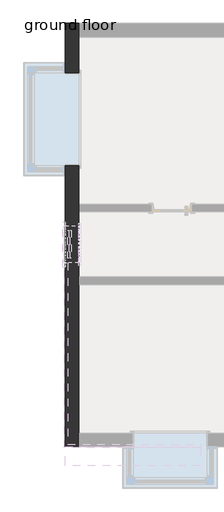
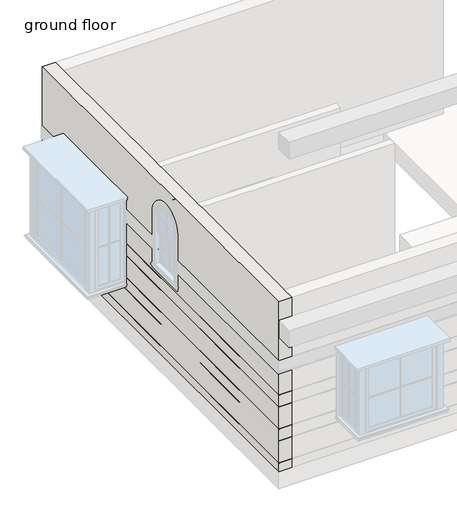
# One storey, part 2 of 5: 1 wall.
"""IFC4 building model written with IfcOpenShell, lengths in millimetres."""

from ifc_helpers import new_model, si_unit, frame, origin, place, context, project, spatial, polyline, circle_curve, ellipse_curve, element, save
from ifc_brep_helpers import plane_surface, cylinder_surface, revolved_surface, advanced_brep

model = new_model("IFC4")

# Units and contexts
model_context = context("Model", 3, world=origin())
ifc_project = project(units=[si_unit("LENGTHUNIT", "METRE", prefix="MILLI")], contexts=[model_context])

# Site, building, storey
site = spatial("IfcSite", under=ifc_project)
building = spatial("IfcBuilding", under=site)
storey = spatial("IfcBuildingStorey", under=building, Name="ground floor", Elevation=304.8)

# Wall
placement = place(None, origin())
element("IfcWall", 1, ObjectType="OUTER WALL 9\"", at=placement, inside=storey, context=model_context, shape_type="AdvancedBrep", body=[
    advanced_brep(
    [(-13179.0672301, -305.6302427, 304.8), (-13179.0672301, -7265.2302427, 304.8), (-13179.0672301, -7265.2302427, 455.95311), (-13179.0672301, -305.6302427, 455.95311), (-13179.0672301, -7265.2302427, 3352.8), (-13179.0672301, -305.6302427, 3352.8), (-13179.0672301, -305.6302427, 2298.7), (-13179.0672301, -1118.4302427, 2298.7), (-13179.0672301, -1118.4302427, 2489.2), (-13179.0672301, -2642.4302427, 2489.2), (-13179.0672301, -2642.4302427, 2298.7), (-13179.0672301, -3633.0302427, 2298.7), (-13179.0672301, -3633.0302427, 2743.2), (-13179.0672301, -4242.6302427, 2743.2), (-13179.0672301, -4242.6302427, 2298.7), (-13179.0672301, -7265.2302427, 2298.7), (-13179.0672301, -2642.4302427, 914.4), (-13179.0672301, -1118.4302427, 914.4), (-13179.0672301, -1118.4302427, 1065.55311), (-13179.0672301, -305.6302427, 1065.55311), (-13179.0672301, -305.6302427, 864.84689), (-13179.0672301, -1118.4302427, 864.84689), (-13179.0672301, -1118.4302427, 850.9), (-13179.0672301, -305.6302427, 850.9), (-13179.0672301, -305.6302427, 469.9), (-13179.0672301, -7265.2302427, 469.9), (-13179.0672301, -7265.2302427, 850.9), (-13179.0672301, -2642.4302427, 850.9), (-13179.0672301, -2642.4302427, 864.84689), (-13179.0672301, -7265.2302427, 864.84689), (-13179.0672301, -7265.2302427, 1065.55311), (-13179.0672301, -2642.4302427, 1065.55311), (-13179.0672301, -4242.6302427, 1828.8), (-13179.0672301, -3633.0302427, 1828.8), (-13179.0672301, -3633.0302427, 2070.1), (-13179.0672301, -2642.4302427, 2070.1), (-13179.0672301, -2642.4302427, 1689.1), (-13179.0672301, -7265.2302427, 1689.1), (-13179.0672301, -7265.2302427, 2070.1), (-13179.0672301, -4242.6302427, 2070.1), (-13179.0672301, -305.6302427, 2284.75311), (-13179.0672301, -305.6302427, 2084.04689), (-13179.0672301, -1118.4302427, 2084.04689), (-13179.0672301, -1118.4302427, 2284.75311), (-13179.0672301, -2642.4302427, 2284.75311), (-13179.0672301, -2642.4302427, 2084.04689), (-13179.0672301, -3633.0302427, 2084.04689), (-13179.0672301, -3633.0302427, 2284.75311), (-13179.0672301, -4242.6302427, 2284.75311), (-13179.0672301, -4242.6302427, 2084.04689), (-13179.0672301, -7265.2302427, 2084.04689), (-13179.0672301, -7265.2302427, 2284.75311), (-13179.0672301, -1118.4302427, 2070.1), (-13179.0672301, -305.6302427, 2070.1), (-13179.0672301, -305.6302427, 1689.1), (-13179.0672301, -1118.4302427, 1689.1), (-13179.0672301, -2642.4302427, 1675.15311), (-13179.0672301, -2642.4302427, 1474.44689), (-13179.0672301, -7265.2302427, 1474.44689), (-13179.0672301, -7265.2302427, 1675.15311), (-13179.0672301, -1118.4302427, 1474.44689), (-13179.0672301, -1118.4302427, 1675.15311), (-13179.0672301, -305.6302427, 1675.15311), (-13179.0672301, -305.6302427, 1474.44689), (-13179.0672301, -7265.2302427, 1460.5), (-13179.0672301, -2642.4302427, 1460.5), (-13179.0672301, -2642.4302427, 1079.5), (-13179.0672301, -7265.2302427, 1079.5), (-13179.0672301, -1118.4302427, 1460.5), (-13179.0672301, -305.6302427, 1460.5), (-13179.0672301, -305.6302427, 1079.5), (-13179.0672301, -1118.4302427, 1079.5), (-12950.4672301, -7265.2302427, 304.8), (-12950.4672301, -7036.6302427, 304.8), (-12950.4672301, -4598.2302427, 304.8), (-12950.4672301, -4471.2302427, 304.8), (-12950.4672301, -3404.4302427, 304.8), (-12950.4672301, -3277.4302427, 304.8), (-12950.4672301, -534.2302427, 304.8), (-12950.4672301, -305.6302427, 304.8), (-12950.4672301, -305.6302427, 3352.8), (-12950.4672301, -534.2302427, 3352.8), (-12950.4672301, -3277.4302427, 3352.8), (-12950.4672301, -3404.4302427, 3352.8), (-12950.4672301, -4471.2302427, 3352.8), (-12950.4672301, -4598.2302427, 3352.8), (-12950.4672301, -7036.6302427, 3352.8), (-12950.4672301, -7265.2302427, 3352.8), (-12950.4672301, -7265.2302427, 2298.7), (-12950.4672301, -7216.8686427, 2298.7), (-12950.4672301, -7216.8686427, 2297.3203242), (-12950.4672301, -7221.2514519, 2292.1465897), (-12950.4672301, -7264.1100243, 2285.00348), (-12950.4672301, -7265.2302427, 2284.75311), (-12950.4672301, -7265.2302427, 2084.04689), (-12950.4672301, -7264.1100243, 2083.79652), (-12950.4672301, -7221.2514519, 2076.6534103), (-12950.4672301, -7216.8686427, 2071.4796758), (-12950.4672301, -7216.8686427, 2070.1), (-12950.4672301, -7265.2302427, 2070.1), (-12950.4672301, -7265.2302427, 1689.1), (-12950.4672301, -7216.8686427, 1689.1), (-12950.4672301, -7216.8686427, 1687.7203242), (-12950.4672301, -7221.2514519, 1682.5465897), (-12950.4672301, -7264.1100243, 1675.40348), (-12950.4672301, -7265.2302427, 1675.15311), (-12950.4672301, -7265.2302427, 1474.44689), (-12950.4672301, -7264.1100243, 1474.19652), (-12950.4672301, -7221.2514519, 1467.0534103), (-12950.4672301, -7216.8686427, 1461.8796758), (-12950.4672301, -7216.8686427, 1460.5), (-12950.4672301, -7265.2302427, 1460.5), (-12950.4672301, -7265.2302427, 1079.5), (-12950.4672301, -7216.8686427, 1079.5), (-12950.4672301, -7216.8686427, 1078.1203242), (-12950.4672301, -7221.2514519, 1072.9465897), (-12950.4672301, -7264.1100243, 1065.80348), (-12950.4672301, -7265.2302427, 1065.55311), (-12950.4672301, -7265.2302427, 864.84689), (-12950.4672301, -7264.1100243, 864.59652), (-12950.4672301, -7221.2514519, 857.4534103), (-12950.4672301, -7216.8686427, 852.2796758), (-12950.4672301, -7216.8686427, 850.9), (-12950.4672301, -7265.2302427, 850.9), (-12950.4672301, -7265.2302427, 469.9), (-12950.4672301, -7216.8686427, 469.9), (-12950.4672301, -7216.8686427, 468.5203242), (-12950.4672301, -7221.2514519, 463.3465897), (-12950.4672301, -7264.1100243, 456.20348), (-12950.4672301, -7265.2302427, 455.95311), (-12950.4672301, -1118.4302427, 2489.2), (-12950.4672301, -1118.4302427, 914.4), (-12950.4672301, -2642.4302427, 914.4), (-12950.4672301, -2642.4302427, 2489.2), (-12950.4672301, -4242.6302427, 2743.2), (-12950.4672301, -3633.0302427, 2743.2), (-12950.4672301, -3633.0302427, 1828.8), (-12950.4672301, -4242.6302427, 1828.8), (-13177.9470117, -305.6302427, 456.20348), (-13135.0884393, -305.6302427, 463.3465897), (-13130.7056301, -305.6302427, 468.5203242), (-13130.7056301, -305.6302427, 469.9), (-13130.7056301, -305.6302427, 850.9), (-13130.7056301, -305.6302427, 852.2796758), (-13135.0884393, -305.6302427, 857.4534103), (-13177.9470117, -305.6302427, 864.59652), (-13177.9470117, -305.6302427, 1065.80348), (-13135.0884393, -305.6302427, 1072.9465897), (-13130.7056301, -305.6302427, 1078.1203242), (-13130.7056301, -305.6302427, 1079.5), (-13130.7056301, -305.6302427, 1460.5), (-13130.7056301, -305.6302427, 1461.8796758), (-13135.0884393, -305.6302427, 1467.0534103), (-13177.9470117, -305.6302427, 1474.19652), (-13177.9470117, -305.6302427, 1675.40348), (-13135.0884393, -305.6302427, 1682.5465897), (-13130.7056301, -305.6302427, 1687.7203242), (-13130.7056301, -305.6302427, 1689.1), (-13130.7056301, -305.6302427, 2070.1), (-13130.7056301, -305.6302427, 2071.4796758), (-13135.0884393, -305.6302427, 2076.6534103), (-13177.9470117, -305.6302427, 2083.79652), (-13177.9470117, -305.6302427, 2285.00348), (-13135.0884393, -305.6302427, 2292.1465897), (-13130.7056301, -305.6302427, 2297.3203242), (-13130.7056301, -305.6302427, 2298.7), (-13130.7056301, -1118.4302427, 2298.7), (-13130.7056301, -1118.4302427, 2297.3203242), (-13135.0884393, -1118.4302427, 2292.1465897), (-13177.9470117, -1118.4302427, 2285.00348), (-13177.9470117, -1118.4302427, 2083.79652), (-13135.0884393, -1118.4302427, 2076.6534103), (-13130.7056301, -1118.4302427, 2071.4796758), (-13130.7056301, -1118.4302427, 2070.1), (-13130.7056301, -1118.4302427, 1689.1), (-13130.7056301, -1118.4302427, 1687.7203242), (-13135.0884393, -1118.4302427, 1682.5465897), (-13177.9470117, -1118.4302427, 1675.40348), (-13177.9470117, -1118.4302427, 1474.19652), (-13135.0884393, -1118.4302427, 1467.0534103), (-13130.7056301, -1118.4302427, 1461.8796758), (-13130.7056301, -1118.4302427, 1460.5), (-13130.7056301, -1118.4302427, 1079.5), (-13130.7056301, -1118.4302427, 1078.1203242), (-13135.0884393, -1118.4302427, 1072.9465897), (-13177.9470117, -1118.4302427, 1065.80348), (-13177.9470117, -2642.4302427, 1065.80348), (-13135.0884393, -2642.4302427, 1072.9465897), (-13130.7056301, -2642.4302427, 1078.1203242), (-13130.7056301, -2642.4302427, 1079.5), (-13130.7056301, -2642.4302427, 1460.5), (-13130.7056301, -2642.4302427, 1461.8796758), (-13135.0884393, -2642.4302427, 1467.0534103), (-13177.9470117, -2642.4302427, 1474.19652), (-13177.9470117, -2642.4302427, 1675.40348), (-13135.0884393, -2642.4302427, 1682.5465897), (-13130.7056301, -2642.4302427, 1687.7203242), (-13130.7056301, -2642.4302427, 1689.1), (-13130.7056301, -2642.4302427, 2070.1), (-13130.7056301, -2642.4302427, 2071.4796758), (-13135.0884393, -2642.4302427, 2076.6534103), (-13177.9470117, -2642.4302427, 2083.79652), (-13177.9470117, -2642.4302427, 2285.00348), (-13135.0884393, -2642.4302427, 2292.1465897), (-13130.7056301, -2642.4302427, 2297.3203242), (-13130.7056301, -2642.4302427, 2298.7), (-13130.7056301, -4242.6302427, 2070.1), (-13130.7056301, -4242.6302427, 2071.4796758), (-13135.0884393, -4242.6302427, 2076.6534103), (-13177.9470117, -4242.6302427, 2083.79652), (-13177.9470117, -4242.6302427, 2285.00348), (-13135.0884393, -4242.6302427, 2292.1465897), (-13130.7056301, -4242.6302427, 2297.3203242), (-13130.7056301, -4242.6302427, 2298.7), (-13130.7056301, -3633.0302427, 2298.7), (-13130.7056301, -3633.0302427, 2297.3203242), (-13135.0884393, -3633.0302427, 2292.1465897), (-13177.9470117, -3633.0302427, 2285.00348), (-13177.9470117, -3633.0302427, 2083.79652), (-13135.0884393, -3633.0302427, 2076.6534103), (-13130.7056301, -3633.0302427, 2071.4796758), (-13130.7056301, -3633.0302427, 2070.1), (-13130.7056301, -7216.8686427, 2298.7), (-13130.7056301, -7216.8686427, 2297.3203242), (-13135.0884393, -7221.2514519, 2292.1465897), (-13177.9470117, -7264.1100243, 2285.00348), (-13177.9470117, -7264.1100243, 2083.79652), (-13135.0884393, -7221.2514519, 2076.6534103), (-13130.7056301, -7216.8686427, 2071.4796758), (-13130.7056301, -7216.8686427, 2070.1), (-13130.7056301, -7216.8686427, 1689.1), (-13130.7056301, -7216.8686427, 1687.7203242), (-13135.0884393, -7221.2514519, 1682.5465897), (-13177.9470117, -7264.1100243, 1675.40348), (-13177.9470117, -7264.1100243, 1474.19652), (-13135.0884393, -7221.2514519, 1467.0534103), (-13130.7056301, -7216.8686427, 1461.8796758), (-13130.7056301, -7216.8686427, 1460.5), (-13135.0884393, -2642.4302427, 857.4534103), (-13177.9470117, -2642.4302427, 864.59652), (-13130.7056301, -2642.4302427, 850.9), (-13130.7056301, -2642.4302427, 852.2796758), (-13130.7056301, -7216.8686427, 1079.5), (-13130.7056301, -7216.8686427, 1078.1203242), (-13135.0884393, -7221.2514519, 1072.9465897), (-13177.9470117, -7264.1100243, 1065.80348), (-13177.9470117, -7264.1100243, 864.59652), (-13135.0884393, -7221.2514519, 857.4534103), (-13130.7056301, -7216.8686427, 852.2796758), (-13130.7056301, -7216.8686427, 850.9), (-13130.7056301, -1118.4302427, 852.2796758), (-13130.7056301, -1118.4302427, 850.9), (-13177.9470117, -1118.4302427, 864.59652), (-13135.0884393, -1118.4302427, 857.4534103), (-13130.7056301, -7216.8686427, 469.9), (-13130.7056301, -7216.8686427, 468.5203242), (-13135.0884393, -7221.2514519, 463.3465897), (-13177.9470117, -7264.1100243, 456.20348)],
    [
        (0, 1),
        (1, 2),
        (2, 3),
        (3, 0),
        (4, 5),
        (5, 6),
        (6, 7),
        (7, 8),
        (8, 9),
        (9, 10),
        (10, 11),
        (11, 12),
        (12, 13, circle_curve(frame((-13179.0672301, -3937.8302427, 2743.2), z_axis=(1.0, 0.0, 0.0), x_axis=(0.0, 1.0, 0.0)), 304.8)),
        (13, 14),
        (14, 15),
        (15, 4),
        (16, 17),
        (17, 18),
        (18, 19),
        (19, 20),
        (20, 21),
        (21, 22),
        (22, 23),
        (23, 24),
        (24, 25),
        (25, 26),
        (26, 27),
        (27, 28),
        (28, 29),
        (29, 30),
        (30, 31),
        (31, 16),
        (32, 33),
        (33, 34),
        (34, 35),
        (35, 36),
        (36, 37),
        (37, 38),
        (38, 39),
        (39, 32),
        (40, 41),
        (41, 42),
        (42, 43),
        (43, 40),
        (44, 45),
        (45, 46),
        (46, 47),
        (47, 44),
        (48, 49),
        (49, 50),
        (50, 51),
        (51, 48),
        (52, 53),
        (53, 54),
        (54, 55),
        (55, 52),
        (56, 57),
        (57, 58),
        (58, 59),
        (59, 56),
        (60, 61),
        (61, 62),
        (62, 63),
        (63, 60),
        (64, 65),
        (65, 66),
        (66, 67),
        (67, 64),
        (68, 69),
        (69, 70),
        (70, 71),
        (71, 68),
        (72, 73),
        (73, 74),
        (74, 75),
        (75, 76),
        (76, 77),
        (77, 78),
        (78, 79),
        (79, 80),
        (80, 81),
        (81, 82),
        (82, 83),
        (83, 84),
        (84, 85),
        (85, 86),
        (86, 87),
        (87, 88),
        (88, 89),
        (89, 90),
        (90, 91, circle_curve(frame((-12950.4672301, -7222.1137427, 2297.3203242), z_axis=(-1.0, 0.0, 0.0), x_axis=(0.0, 1.0, 0.0)), 5.2451)),
        (91, 92),
        (92, 93, circle_curve(frame((-12950.4672301, -7262.3854427, 2274.656011), z_axis=(1.0, 0.0, 0.0), x_axis=(0.0, 1.0, 0.0)), 10.4902)),
        (93, 94),
        (94, 95, circle_curve(frame((-12950.4672301, -7262.3854427, 2094.143989), z_axis=(1.0, 0.0, 0.0), x_axis=(0.0, 1.0, 0.0)), 10.4902)),
        (95, 96),
        (96, 97, circle_curve(frame((-12950.4672301, -7222.1137427, 2071.4796758), z_axis=(-1.0, 0.0, 0.0), x_axis=(0.0, 1.0, 0.0)), 5.2451)),
        (97, 98),
        (98, 99),
        (99, 100),
        (100, 101),
        (101, 102),
        (102, 103, circle_curve(frame((-12950.4672301, -7222.1137427, 1687.7203242), z_axis=(-1.0, 0.0, 0.0), x_axis=(0.0, 1.0, 0.0)), 5.2451)),
        (103, 104),
        (104, 105, circle_curve(frame((-12950.4672301, -7262.3854427, 1665.056011), z_axis=(1.0, 0.0, 0.0), x_axis=(0.0, 1.0, 0.0)), 10.4902)),
        (105, 106),
        (106, 107, circle_curve(frame((-12950.4672301, -7262.3854427, 1484.543989), z_axis=(1.0, 0.0, 0.0), x_axis=(0.0, 1.0, 0.0)), 10.4902)),
        (107, 108),
        (108, 109, circle_curve(frame((-12950.4672301, -7222.1137427, 1461.8796758), z_axis=(-1.0, 0.0, 0.0), x_axis=(0.0, 1.0, 0.0)), 5.2451)),
        (109, 110),
        (110, 111),
        (111, 112),
        (112, 113),
        (113, 114),
        (114, 115, circle_curve(frame((-12950.4672301, -7222.1137427, 1078.1203242), z_axis=(-1.0, 0.0, 0.0), x_axis=(0.0, 1.0, 0.0)), 5.2451)),
        (115, 116),
        (116, 117, circle_curve(frame((-12950.4672301, -7262.3854427, 1055.456011), z_axis=(1.0, 0.0, 0.0), x_axis=(0.0, 1.0, 0.0)), 10.4902)),
        (117, 118),
        (118, 119, circle_curve(frame((-12950.4672301, -7262.3854427, 874.943989), z_axis=(1.0, 0.0, 0.0), x_axis=(0.0, 1.0, 0.0)), 10.4902)),
        (119, 120),
        (120, 121, circle_curve(frame((-12950.4672301, -7222.1137427, 852.2796758), z_axis=(-1.0, 0.0, 0.0), x_axis=(0.0, 1.0, 0.0)), 5.2451)),
        (121, 122),
        (122, 123),
        (123, 124),
        (124, 125),
        (125, 126),
        (126, 127, circle_curve(frame((-12950.4672301, -7222.1137427, 468.5203242), z_axis=(-1.0, 0.0, 0.0), x_axis=(0.0, 1.0, 0.0)), 5.2451)),
        (127, 128),
        (128, 129, circle_curve(frame((-12950.4672301, -7262.3854427, 445.856011), z_axis=(1.0, 0.0, 0.0), x_axis=(0.0, 1.0, 0.0)), 10.4902)),
        (129, 72),
        (130, 131),
        (131, 132),
        (132, 133),
        (133, 130),
        (134, 135, circle_curve(frame((-12950.4672301, -3937.8302427, 2743.2), z_axis=(-1.0, 0.0, 0.0), x_axis=(0.0, 1.0, 0.0)), 304.8)),
        (135, 136),
        (136, 137),
        (137, 134),
        (0, 79),
        (72, 1),
        (4, 87),
        (80, 5),
        (129, 2),
        (15, 88),
        (99, 38),
        (37, 100),
        (93, 51),
        (50, 94),
        (111, 64),
        (67, 112),
        (105, 59),
        (58, 106),
        (123, 26),
        (25, 124),
        (117, 30),
        (29, 118),
        (3, 138, circle_curve(frame((-13176.2224301, -305.6302427, 445.856011), z_axis=(0.0, 1.0, 0.0), x_axis=(1.0, 0.0, 0.0)), 10.4902)),
        (138, 139),
        (139, 140, circle_curve(frame((-13135.9507301, -305.6302427, 468.5203242), z_axis=(0.0, -1.0, 0.0), x_axis=(1.0, 0.0, 0.0)), 5.2451)),
        (140, 141),
        (141, 24),
        (23, 142),
        (142, 143),
        (143, 144, circle_curve(frame((-13135.9507301, -305.6302427, 852.2796758), z_axis=(0.0, -1.0, 0.0), x_axis=(1.0, 0.0, 0.0)), 5.2451)),
        (144, 145),
        (145, 20, circle_curve(frame((-13176.2224301, -305.6302427, 874.943989), z_axis=(0.0, 1.0, 0.0), x_axis=(1.0, 0.0, 0.0)), 10.4902)),
        (19, 146, circle_curve(frame((-13176.2224301, -305.6302427, 1055.456011), z_axis=(0.0, 1.0, 0.0), x_axis=(1.0, 0.0, 0.0)), 10.4902)),
        (146, 147),
        (147, 148, circle_curve(frame((-13135.9507301, -305.6302427, 1078.1203242), z_axis=(0.0, -1.0, 0.0), x_axis=(1.0, 0.0, 0.0)), 5.2451)),
        (148, 149),
        (149, 70),
        (69, 150),
        (150, 151),
        (151, 152, circle_curve(frame((-13135.9507301, -305.6302427, 1461.8796758), z_axis=(0.0, -1.0, 0.0), x_axis=(1.0, 0.0, 0.0)), 5.2451)),
        (152, 153),
        (153, 63, circle_curve(frame((-13176.2224301, -305.6302427, 1484.543989), z_axis=(0.0, 1.0, 0.0), x_axis=(1.0, 0.0, 0.0)), 10.4902)),
        (62, 154, circle_curve(frame((-13176.2224301, -305.6302427, 1665.056011), z_axis=(0.0, 1.0, 0.0), x_axis=(1.0, 0.0, 0.0)), 10.4902)),
        (154, 155),
        (155, 156, circle_curve(frame((-13135.9507301, -305.6302427, 1687.7203242), z_axis=(0.0, -1.0, 0.0), x_axis=(1.0, 0.0, 0.0)), 5.2451)),
        (156, 157),
        (157, 54),
        (53, 158),
        (158, 159),
        (159, 160, circle_curve(frame((-13135.9507301, -305.6302427, 2071.4796758), z_axis=(0.0, -1.0, 0.0), x_axis=(1.0, 0.0, 0.0)), 5.2451)),
        (160, 161),
        (161, 41, circle_curve(frame((-13176.2224301, -305.6302427, 2094.143989), z_axis=(0.0, 1.0, 0.0), x_axis=(1.0, 0.0, 0.0)), 10.4902)),
        (40, 162, circle_curve(frame((-13176.2224301, -305.6302427, 2274.656011), z_axis=(0.0, 1.0, 0.0), x_axis=(1.0, 0.0, 0.0)), 10.4902)),
        (162, 163),
        (163, 164, circle_curve(frame((-13135.9507301, -305.6302427, 2297.3203242), z_axis=(0.0, -1.0, 0.0), x_axis=(1.0, 0.0, 0.0)), 5.2451)),
        (164, 165),
        (165, 6),
        (130, 8),
        (7, 166),
        (166, 167),
        (167, 168, circle_curve(frame((-13135.9507301, -1118.4302427, 2297.3203242), z_axis=(0.0, 1.0, 0.0), x_axis=(1.0, 0.0, 0.0)), 5.2451)),
        (168, 169),
        (169, 43, circle_curve(frame((-13176.2224301, -1118.4302427, 2274.656011), z_axis=(0.0, -1.0, 0.0), x_axis=(1.0, 0.0, 0.0)), 10.4902)),
        (42, 170, circle_curve(frame((-13176.2224301, -1118.4302427, 2094.143989), z_axis=(0.0, -1.0, 0.0), x_axis=(1.0, 0.0, 0.0)), 10.4902)),
        (170, 171),
        (171, 172, circle_curve(frame((-13135.9507301, -1118.4302427, 2071.4796758), z_axis=(0.0, 1.0, 0.0), x_axis=(1.0, 0.0, 0.0)), 5.2451)),
        (172, 173),
        (173, 52),
        (55, 174),
        (174, 175),
        (175, 176, circle_curve(frame((-13135.9507301, -1118.4302427, 1687.7203242), z_axis=(0.0, 1.0, 0.0), x_axis=(1.0, 0.0, 0.0)), 5.2451)),
        (176, 177),
        (177, 61, circle_curve(frame((-13176.2224301, -1118.4302427, 1665.056011), z_axis=(0.0, -1.0, 0.0), x_axis=(1.0, 0.0, 0.0)), 10.4902)),
        (60, 178, circle_curve(frame((-13176.2224301, -1118.4302427, 1484.543989), z_axis=(0.0, -1.0, 0.0), x_axis=(1.0, 0.0, 0.0)), 10.4902)),
        (178, 179),
        (179, 180, circle_curve(frame((-13135.9507301, -1118.4302427, 1461.8796758), z_axis=(0.0, 1.0, 0.0), x_axis=(1.0, 0.0, 0.0)), 5.2451)),
        (180, 181),
        (181, 68),
        (71, 182),
        (182, 183),
        (183, 184, circle_curve(frame((-13135.9507301, -1118.4302427, 1078.1203242), z_axis=(0.0, 1.0, 0.0), x_axis=(1.0, 0.0, 0.0)), 5.2451)),
        (184, 185),
        (185, 18, circle_curve(frame((-13176.2224301, -1118.4302427, 1055.456011), z_axis=(0.0, -1.0, 0.0), x_axis=(1.0, 0.0, 0.0)), 10.4902)),
        (17, 131),
        (16, 132),
        (31, 186, circle_curve(frame((-13176.2224301, -2642.4302427, 1055.456011), z_axis=(0.0, 1.0, 0.0), x_axis=(1.0, 0.0, 0.0)), 10.4902)),
        (186, 187),
        (187, 188, circle_curve(frame((-13135.9507301, -2642.4302427, 1078.1203242), z_axis=(0.0, -1.0, 0.0), x_axis=(1.0, 0.0, 0.0)), 5.2451)),
        (188, 189),
        (189, 66),
        (65, 190),
        (190, 191),
        (191, 192, circle_curve(frame((-13135.9507301, -2642.4302427, 1461.8796758), z_axis=(0.0, -1.0, 0.0), x_axis=(1.0, 0.0, 0.0)), 5.2451)),
        (192, 193),
        (193, 57, circle_curve(frame((-13176.2224301, -2642.4302427, 1484.543989), z_axis=(0.0, 1.0, 0.0), x_axis=(1.0, 0.0, 0.0)), 10.4902)),
        (56, 194, circle_curve(frame((-13176.2224301, -2642.4302427, 1665.056011), z_axis=(0.0, 1.0, 0.0), x_axis=(1.0, 0.0, 0.0)), 10.4902)),
        (194, 195),
        (195, 196, circle_curve(frame((-13135.9507301, -2642.4302427, 1687.7203242), z_axis=(0.0, -1.0, 0.0), x_axis=(1.0, 0.0, 0.0)), 5.2451)),
        (196, 197),
        (197, 36),
        (35, 198),
        (198, 199),
        (199, 200, circle_curve(frame((-13135.9507301, -2642.4302427, 2071.4796758), z_axis=(0.0, -1.0, 0.0), x_axis=(1.0, 0.0, 0.0)), 5.2451)),
        (200, 201),
        (201, 45, circle_curve(frame((-13176.2224301, -2642.4302427, 2094.143989), z_axis=(0.0, 1.0, 0.0), x_axis=(1.0, 0.0, 0.0)), 10.4902)),
        (44, 202, circle_curve(frame((-13176.2224301, -2642.4302427, 2274.656011), z_axis=(0.0, 1.0, 0.0), x_axis=(1.0, 0.0, 0.0)), 10.4902)),
        (202, 203),
        (203, 204, circle_curve(frame((-13135.9507301, -2642.4302427, 2297.3203242), z_axis=(0.0, -1.0, 0.0), x_axis=(1.0, 0.0, 0.0)), 5.2451)),
        (204, 205),
        (205, 10),
        (9, 133),
        (12, 135),
        (134, 13),
        (137, 32),
        (39, 206),
        (206, 207),
        (207, 208, circle_curve(frame((-13135.9507301, -4242.6302427, 2071.4796758), z_axis=(0.0, -1.0, 0.0), x_axis=(1.0, 0.0, 0.0)), 5.2451)),
        (208, 209),
        (209, 49, circle_curve(frame((-13176.2224301, -4242.6302427, 2094.143989), z_axis=(0.0, 1.0, 0.0), x_axis=(1.0, 0.0, 0.0)), 10.4902)),
        (48, 210, circle_curve(frame((-13176.2224301, -4242.6302427, 2274.656011), z_axis=(0.0, 1.0, 0.0), x_axis=(1.0, 0.0, 0.0)), 10.4902)),
        (210, 211),
        (211, 212, circle_curve(frame((-13135.9507301, -4242.6302427, 2297.3203242), z_axis=(0.0, -1.0, 0.0), x_axis=(1.0, 0.0, 0.0)), 5.2451)),
        (212, 213),
        (213, 14),
        (136, 33),
        (11, 214),
        (214, 215),
        (215, 216, circle_curve(frame((-13135.9507301, -3633.0302427, 2297.3203242), z_axis=(0.0, 1.0, 0.0), x_axis=(1.0, 0.0, 0.0)), 5.2451)),
        (216, 217),
        (217, 47, circle_curve(frame((-13176.2224301, -3633.0302427, 2274.656011), z_axis=(0.0, -1.0, 0.0), x_axis=(1.0, 0.0, 0.0)), 10.4902)),
        (46, 218, circle_curve(frame((-13176.2224301, -3633.0302427, 2094.143989), z_axis=(0.0, -1.0, 0.0), x_axis=(1.0, 0.0, 0.0)), 10.4902)),
        (218, 219),
        (219, 220, circle_curve(frame((-13135.9507301, -3633.0302427, 2071.4796758), z_axis=(0.0, 1.0, 0.0), x_axis=(1.0, 0.0, 0.0)), 5.2451)),
        (220, 221),
        (221, 34),
        (213, 222),
        (222, 89),
        (212, 223),
        (223, 222),
        (211, 224),
        (224, 223, ellipse_curve(frame((-13135.9507301, -7222.1137427, 2297.3203242), z_axis=(0.7071067811865458, -0.7071067811865492, 0.0), x_axis=(0.7071067811865492, 0.7071067811865458, 0.0)), 7.4176916, 5.2451)),
        (210, 225),
        (225, 224),
        (51, 225, ellipse_curve(frame((-13176.2224301, -7262.3854427, 2274.656011), z_axis=(-0.7071067811865458, 0.7071067811865492, 0.0), x_axis=(-0.7071067811865492, -0.7071067811865458, 0.0)), 14.8353831, 10.4902)),
        (209, 226),
        (226, 50, ellipse_curve(frame((-13176.2224301, -7262.3854427, 2094.143989), z_axis=(-0.7071067811865458, 0.7071067811865492, 0.0), x_axis=(-0.7071067811865492, -0.7071067811865458, 0.0)), 14.8353831, 10.4902)),
        (208, 227),
        (227, 226),
        (207, 228),
        (228, 227, ellipse_curve(frame((-13135.9507301, -7222.1137427, 2071.4796758), z_axis=(0.7071067811865458, -0.7071067811865492, 0.0), x_axis=(0.7071067811865492, 0.7071067811865458, 0.0)), 7.4176916, 5.2451)),
        (206, 229),
        (229, 228),
        (98, 229),
        (223, 90),
        (224, 91),
        (225, 92),
        (226, 95),
        (227, 96),
        (228, 97),
        (205, 214),
        (204, 215),
        (203, 216),
        (202, 217),
        (201, 218),
        (200, 219),
        (199, 220),
        (198, 221),
        (165, 166),
        (164, 167),
        (163, 168),
        (162, 169),
        (161, 170),
        (160, 171),
        (159, 172),
        (158, 173),
        (197, 230),
        (230, 101),
        (196, 231),
        (231, 230),
        (195, 232),
        (232, 231, ellipse_curve(frame((-13135.9507301, -7222.1137427, 1687.7203242), z_axis=(0.707106781186546, -0.707106781186549, 0.0), x_axis=(0.707106781186549, 0.707106781186546, 0.0)), 7.4176916, 5.2451)),
        (194, 233),
        (233, 232),
        (59, 233, ellipse_curve(frame((-13176.2224301, -7262.3854427, 1665.056011), z_axis=(-0.707106781186546, 0.707106781186549, 0.0), x_axis=(-0.707106781186549, -0.707106781186546, 0.0)), 14.8353831, 10.4902)),
        (193, 234),
        (234, 58, ellipse_curve(frame((-13176.2224301, -7262.3854427, 1484.543989), z_axis=(-0.707106781186546, 0.707106781186549, 0.0), x_axis=(-0.707106781186549, -0.707106781186546, 0.0)), 14.8353831, 10.4902)),
        (192, 235),
        (235, 234),
        (191, 236),
        (236, 235, ellipse_curve(frame((-13135.9507301, -7222.1137427, 1461.8796758), z_axis=(0.707106781186546, -0.707106781186549, 0.0), x_axis=(0.707106781186549, 0.707106781186546, 0.0)), 7.4176916, 5.2451)),
        (190, 237),
        (237, 236),
        (110, 237),
        (231, 102),
        (232, 103),
        (233, 104),
        (234, 107),
        (235, 108),
        (236, 109),
        (157, 174),
        (156, 175),
        (155, 176),
        (154, 177),
        (153, 178),
        (152, 179),
        (151, 180),
        (150, 181),
        (238, 239),
        (239, 28, circle_curve(frame((-13176.2224301, -2642.4302427, 874.943989), z_axis=(0.0, 1.0, 0.0), x_axis=(1.0, 0.0, 0.0)), 10.4902)),
        (27, 240),
        (240, 241),
        (241, 238, circle_curve(frame((-13135.9507301, -2642.4302427, 852.2796758), z_axis=(0.0, -1.0, 0.0), x_axis=(1.0, 0.0, 0.0)), 5.2451)),
        (189, 242),
        (242, 113),
        (188, 243),
        (243, 242),
        (187, 244),
        (244, 243, ellipse_curve(frame((-13135.9507301, -7222.1137427, 1078.1203242), z_axis=(0.707106781186546, -0.707106781186549, 0.0), x_axis=(0.707106781186549, 0.707106781186546, 0.0)), 7.4176916, 5.2451)),
        (186, 245),
        (245, 244),
        (30, 245, ellipse_curve(frame((-13176.2224301, -7262.3854427, 1055.456011), z_axis=(-0.707106781186546, 0.707106781186549, 0.0), x_axis=(-0.707106781186549, -0.707106781186546, 0.0)), 14.8353831, 10.4902)),
        (239, 246),
        (246, 29, ellipse_curve(frame((-13176.2224301, -7262.3854427, 874.943989), z_axis=(-0.707106781186546, 0.707106781186549, 0.0), x_axis=(-0.707106781186549, -0.707106781186546, 0.0)), 14.8353831, 10.4902)),
        (238, 247),
        (247, 246),
        (241, 248),
        (248, 247, ellipse_curve(frame((-13135.9507301, -7222.1137427, 852.2796758), z_axis=(0.707106781186546, -0.707106781186549, 0.0), x_axis=(0.707106781186549, 0.707106781186546, 0.0)), 7.4176916, 5.2451)),
        (240, 249),
        (249, 248),
        (122, 249),
        (243, 114),
        (244, 115),
        (245, 116),
        (246, 119),
        (247, 120),
        (248, 121),
        (250, 251),
        (251, 22),
        (21, 252, circle_curve(frame((-13176.2224301, -1118.4302427, 874.943989), z_axis=(0.0, -1.0, 0.0), x_axis=(1.0, 0.0, 0.0)), 10.4902)),
        (252, 253),
        (253, 250, circle_curve(frame((-13135.9507301, -1118.4302427, 852.2796758), z_axis=(0.0, 1.0, 0.0), x_axis=(1.0, 0.0, 0.0)), 5.2451)),
        (149, 182),
        (148, 183),
        (147, 184),
        (146, 185),
        (145, 252),
        (144, 253),
        (143, 250),
        (142, 251),
        (141, 254),
        (254, 125),
        (140, 255),
        (255, 254),
        (139, 256),
        (256, 255, ellipse_curve(frame((-13135.9507301, -7222.1137427, 468.5203242), z_axis=(0.7071067811865458, -0.7071067811865491, 0.0), x_axis=(0.7071067811865489, 0.707106781186546, 0.0)), 7.4176916, 5.2451)),
        (138, 257),
        (257, 256),
        (2, 257, ellipse_curve(frame((-13176.2224301, -7262.3854427, 445.856011), z_axis=(-0.7071067811865458, 0.7071067811865491, 0.0), x_axis=(-0.7071067811865489, -0.707106781186546, 0.0)), 14.8353831, 10.4902)),
        (255, 126),
        (256, 127),
        (257, 128),
    ],
    [
        plane_surface(frame((-13179.0672301, -305.6302427, 304.8), z_axis=(-1.0, 0.0, 0.0), x_axis=(0.0, -1.0, 0.0))),
        plane_surface(frame((-12950.4672301, -305.6302427, 304.8), z_axis=(1.0, 0.0, 0.0), x_axis=(0.0, 1.0, 0.0))),
        plane_surface(frame((-13179.0672301, -419.9302427, 304.8), z_axis=(0.0, 0.0, -1.0), x_axis=(1.0, 0.0, 0.0))),
        plane_surface(frame((-13179.0672301, -7150.9302427, 3352.8), z_axis=(0.0, 0.0, 1.0), x_axis=(1.0, 0.0, 0.0))),
        plane_surface(frame((-13179.0672301, -7265.2302427, 304.8), z_axis=(0.0, -1.0, 0.0), x_axis=(1.0, 0.0, 0.0))),
        plane_surface(frame((-12942.6830845, -305.6302427, 304.8), z_axis=(0.0, 1.0, 0.0), x_axis=(-1.0, 0.0, 0.0))),
        plane_surface(frame((-12950.4672301, -1118.4302427, 2489.2), z_axis=(0.0, -1.0, 0.0), x_axis=(-1.0, 0.0, 0.0))),
        plane_surface(frame((-12950.4672301, -1118.4302427, 914.4), z_axis=(0.0, 0.0, 1.0), x_axis=(-1.0, 0.0, 0.0))),
        plane_surface(frame((-12950.4672301, -2642.4302427, 914.4), z_axis=(0.0, 1.0, 0.0), x_axis=(-1.0, 0.0, 0.0))),
        plane_surface(frame((-12950.4672301, -2642.4302427, 2489.2), z_axis=(0.0, 0.0, -1.0), x_axis=(-1.0, 0.0, 0.0))),
        revolved_surface(polyline([(-12950.4672301, -3633.0302426999997, 2743.2), (-13179.0672301, -3633.0302426999997, 2743.2)]), (-12950.4672301, -3937.8302427, 2743.2), (1.0, 0.0, 0.0)),
        plane_surface(frame((-13179.0672301, -4242.6302427, 2743.2), z_axis=(0.0, 1.0, 0.0), x_axis=(1.0, 0.0, 0.0))),
        plane_surface(frame((-13179.0672301, -4242.6302427, 1828.8), z_axis=(0.0, 0.0, 1.0), x_axis=(1.0, 0.0, 0.0))),
        plane_surface(frame((-13179.0672301, -3633.0302427, 1828.8), z_axis=(0.0, -1.0, 0.0), x_axis=(1.0, 0.0, 0.0))),
        plane_surface(frame((-13193.9516301, -4242.6302427, 2298.7), z_axis=(0.0, 0.0, -1.0), x_axis=(0.0, -1.0, 0.0))),
        plane_surface(frame((-13130.7056301, -4242.6302427, 2298.7), z_axis=(-1.0, 0.0, 0.0), x_axis=(0.0, -1.0, 0.0))),
        revolved_surface(polyline([(-13130.7056301, -4242.6302427, 2297.3203242), (-13130.7056301, -7227.358842731111, 2297.3203242)]), (-13135.9507301, -4242.6302427, 2297.3203242), (0.0, 1.0, 0.0)),
        plane_surface(frame((-13158.7091301, -4242.6302427, 2288.2098), z_axis=(-0.16439930721687146, 0.0, 0.9863938705135048), x_axis=(0.0, -1.0, 0.0))),
        cylinder_surface(frame((-13176.2224301, -4242.6302427, 2274.656011), z_axis=(0.0, -1.0, 0.0), x_axis=(1.0, 0.0, 0.0)), 10.4902),
        cylinder_surface(frame((-13176.2224301, -4242.6302427, 2094.143989), z_axis=(0.0, -1.0, 0.0), x_axis=(1.0, 0.0, 0.0)), 10.4902),
        plane_surface(frame((-13158.7091301, -4242.6302427, 2080.5902), z_axis=(-0.16439930721687793, 0.0, -0.9863938705135037), x_axis=(0.0, -1.0, 0.0))),
        revolved_surface(polyline([(-13130.7056301, -4242.6302427, 2071.4796758), (-13130.7056301, -7227.358842731111, 2071.4796758)]), (-13135.9507301, -4242.6302427, 2071.4796758), (0.0, 1.0, 0.0)),
        plane_surface(frame((-13130.7056301, -4242.6302427, 2071.4796758), z_axis=(-1.0, 0.0, 0.0), x_axis=(0.0, -1.0, 0.0))),
        plane_surface(frame((-13130.7056301, -4242.6302427, 2070.1), z_axis=(0.0, 0.0, 1.0), x_axis=(0.0, -1.0, 0.0))),
        plane_surface(frame((-13130.7056301, -7216.8686427, 2298.7), z_axis=(0.0, -1.0, 0.0), x_axis=(1.0, 0.0, 0.0))),
        revolved_surface(polyline([(-13141.19583013111, -7216.8686427, 2297.3203242), (-12950.4672301, -7216.8686427, 2297.3203242)]), (-13179.0672301, -7222.1137427, 2297.3203242), (-1.0, 0.0, 0.0)),
        plane_surface(frame((-13158.7091301, -7244.8721427, 2288.2098), z_axis=(0.0, -0.16439930721687152, 0.9863938705135048), x_axis=(1.0, 0.0, 0.0))),
        cylinder_surface(frame((-13179.0672301, -7262.3854427, 2274.656011), z_axis=(1.0, 0.0, 0.0), x_axis=(0.0, 1.0, 0.0)), 10.4902),
        cylinder_surface(frame((-13179.0672301, -7262.3854427, 2094.143989), z_axis=(1.0, 0.0, 0.0), x_axis=(0.0, 1.0, 0.0)), 10.4902),
        plane_surface(frame((-13158.7091301, -7244.8721427, 2080.5902), z_axis=(0.0, -0.16439930721687793, -0.9863938705135037), x_axis=(1.0, 0.0, 0.0))),
        revolved_surface(polyline([(-13141.19583013111, -7216.8686427, 2071.4796758), (-12950.4672301, -7216.8686427, 2071.4796758)]), (-13179.0672301, -7222.1137427, 2071.4796758), (-1.0, 0.0, 0.0)),
        plane_surface(frame((-13130.7056301, -7216.8686427, 2071.4796758), z_axis=(0.0, -1.0, 0.0), x_axis=(1.0, 0.0, 0.0))),
        plane_surface(frame((-13193.9516301, -2642.4302427, 2298.7), z_axis=(0.0, 0.0, -1.0), x_axis=(0.0, -1.0, 0.0))),
        plane_surface(frame((-13130.7056301, -2642.4302427, 2298.7), z_axis=(-1.0, 0.0, 0.0), x_axis=(0.0, -1.0, 0.0))),
        revolved_surface(polyline([(-13130.7056301, -2642.4302427, 2297.3203242), (-13130.7056301, -3633.0302427, 2297.3203242)]), (-13135.9507301, -2642.4302427, 2297.3203242), (0.0, 1.0, 0.0)),
        plane_surface(frame((-13158.7091301, -2642.4302427, 2288.2098), z_axis=(-0.16439930721687146, 0.0, 0.9863938705135048), x_axis=(0.0, -1.0, 0.0))),
        cylinder_surface(frame((-13176.2224301, -2642.4302427, 2274.656011), z_axis=(0.0, -1.0, 0.0), x_axis=(1.0, 0.0, 0.0)), 10.4902),
        cylinder_surface(frame((-13176.2224301, -2642.4302427, 2094.143989), z_axis=(0.0, -1.0, 0.0), x_axis=(1.0, 0.0, 0.0)), 10.4902),
        plane_surface(frame((-13158.7091301, -2642.4302427, 2080.5902), z_axis=(-0.16439930721687793, 0.0, -0.9863938705135037), x_axis=(0.0, -1.0, 0.0))),
        revolved_surface(polyline([(-13130.7056301, -2642.4302427, 2071.4796758), (-13130.7056301, -3633.0302427, 2071.4796758)]), (-13135.9507301, -2642.4302427, 2071.4796758), (0.0, 1.0, 0.0)),
        plane_surface(frame((-13130.7056301, -2642.4302427, 2071.4796758), z_axis=(-1.0, 0.0, 0.0), x_axis=(0.0, -1.0, 0.0))),
        plane_surface(frame((-13130.7056301, -2642.4302427, 2070.1), z_axis=(0.0, 0.0, 1.0), x_axis=(0.0, -1.0, 0.0))),
        plane_surface(frame((-13193.9516301, -305.6302427, 2298.7), z_axis=(0.0, 0.0, -1.0), x_axis=(0.0, -1.0, 0.0))),
        plane_surface(frame((-13130.7056301, -305.6302427, 2298.7), z_axis=(-1.0, 0.0, 0.0), x_axis=(0.0, -1.0, 0.0))),
        revolved_surface(polyline([(-13130.7056301, -305.6302427, 2297.3203242), (-13130.7056301, -1118.4302427, 2297.3203242)]), (-13135.9507301, -305.6302427, 2297.3203242), (0.0, 1.0, 0.0)),
        plane_surface(frame((-13158.7091301, -305.6302427, 2288.2098), z_axis=(-0.16439930721687146, 0.0, 0.9863938705135048), x_axis=(0.0, -1.0, 0.0))),
        cylinder_surface(frame((-13176.2224301, -305.6302427, 2274.656011), z_axis=(0.0, -1.0, 0.0), x_axis=(1.0, 0.0, 0.0)), 10.4902),
        cylinder_surface(frame((-13176.2224301, -305.6302427, 2094.143989), z_axis=(0.0, -1.0, 0.0), x_axis=(1.0, 0.0, 0.0)), 10.4902),
        plane_surface(frame((-13158.7091301, -305.6302427, 2080.5902), z_axis=(-0.16439930721687793, 0.0, -0.9863938705135037), x_axis=(0.0, -1.0, 0.0))),
        revolved_surface(polyline([(-13130.7056301, -305.6302427, 2071.4796758), (-13130.7056301, -1118.4302427, 2071.4796758)]), (-13135.9507301, -305.6302427, 2071.4796758), (0.0, 1.0, 0.0)),
        plane_surface(frame((-13130.7056301, -305.6302427, 2071.4796758), z_axis=(-1.0, 0.0, 0.0), x_axis=(0.0, -1.0, 0.0))),
        plane_surface(frame((-13130.7056301, -305.6302427, 2070.1), z_axis=(0.0, 0.0, 1.0), x_axis=(0.0, -1.0, 0.0))),
        plane_surface(frame((-13193.9516301, -2642.4302427, 1689.1), z_axis=(0.0, 0.0, -1.0), x_axis=(0.0, -1.0, 0.0))),
        plane_surface(frame((-13130.7056301, -2642.4302427, 1689.1), z_axis=(-1.0, 0.0, 0.0), x_axis=(0.0, -1.0, 0.0))),
        revolved_surface(polyline([(-13130.7056301, -2642.4302427, 1687.7203242), (-13130.7056301, -7227.3588427311115, 1687.7203242)]), (-13135.9507301, -2642.4302427, 1687.7203242), (0.0, 1.0, 0.0)),
        plane_surface(frame((-13158.7091301, -2642.4302427, 1678.6098), z_axis=(-0.16439930721687146, 0.0, 0.9863938705135048), x_axis=(0.0, -1.0, 0.0))),
        cylinder_surface(frame((-13176.2224301, -2642.4302427, 1665.056011), z_axis=(0.0, -1.0, 0.0), x_axis=(1.0, 0.0, 0.0)), 10.4902),
        cylinder_surface(frame((-13176.2224301, -2642.4302427, 1484.543989), z_axis=(0.0, -1.0, 0.0), x_axis=(1.0, 0.0, 0.0)), 10.4902),
        plane_surface(frame((-13158.7091301, -2642.4302427, 1470.9902), z_axis=(-0.16439930721687793, 0.0, -0.9863938705135037), x_axis=(0.0, -1.0, 0.0))),
        revolved_surface(polyline([(-13130.7056301, -2642.4302427, 1461.8796758), (-13130.7056301, -7227.3588427311115, 1461.8796758)]), (-13135.9507301, -2642.4302427, 1461.8796758), (0.0, 1.0, 0.0)),
        plane_surface(frame((-13130.7056301, -2642.4302427, 1461.8796758), z_axis=(-1.0, 0.0, 0.0), x_axis=(0.0, -1.0, 0.0))),
        plane_surface(frame((-13130.7056301, -2642.4302427, 1460.5), z_axis=(0.0, 0.0, 1.0), x_axis=(0.0, -1.0, 0.0))),
        plane_surface(frame((-13130.7056301, -7216.8686427, 1689.1), z_axis=(0.0, -1.0, 0.0), x_axis=(1.0, 0.0, 0.0))),
        revolved_surface(polyline([(-13141.19583013111, -7216.8686427, 1687.7203242), (-12950.4672301, -7216.8686427, 1687.7203242)]), (-13179.0672301, -7222.1137427, 1687.7203242), (-1.0, 0.0, 0.0)),
        plane_surface(frame((-13158.7091301, -7244.8721427, 1678.6098), z_axis=(0.0, -0.1643993072168715, 0.9863938705135048), x_axis=(1.0, 0.0, 0.0))),
        cylinder_surface(frame((-13179.0672301, -7262.3854427, 1665.056011), z_axis=(1.0, 0.0, 0.0), x_axis=(0.0, 1.0, 0.0)), 10.4902),
        cylinder_surface(frame((-13179.0672301, -7262.3854427, 1484.543989), z_axis=(1.0, 0.0, 0.0), x_axis=(0.0, 1.0, 0.0)), 10.4902),
        plane_surface(frame((-13158.7091301, -7244.8721427, 1470.9902), z_axis=(0.0, -0.16439930721687795, -0.9863938705135037), x_axis=(1.0, 0.0, 0.0))),
        revolved_surface(polyline([(-13141.19583013111, -7216.8686427, 1461.8796758), (-12950.4672301, -7216.8686427, 1461.8796758)]), (-13179.0672301, -7222.1137427, 1461.8796758), (-1.0, 0.0, 0.0)),
        plane_surface(frame((-13130.7056301, -7216.8686427, 1461.8796758), z_axis=(0.0, -1.0, 0.0), x_axis=(1.0, 0.0, 0.0))),
        plane_surface(frame((-13193.9516301, -305.6302427, 1689.1), z_axis=(0.0, 0.0, -1.0), x_axis=(0.0, -1.0, 0.0))),
        plane_surface(frame((-13130.7056301, -305.6302427, 1689.1), z_axis=(-1.0, 0.0, 0.0), x_axis=(0.0, -1.0, 0.0))),
        revolved_surface(polyline([(-13130.7056301, -305.6302427, 1687.7203242), (-13130.7056301, -1118.4302427, 1687.7203242)]), (-13135.9507301, -305.6302427, 1687.7203242), (0.0, 1.0, 0.0)),
        plane_surface(frame((-13158.7091301, -305.6302427, 1678.6098), z_axis=(-0.16439930721687146, 0.0, 0.9863938705135048), x_axis=(0.0, -1.0, 0.0))),
        cylinder_surface(frame((-13176.2224301, -305.6302427, 1665.056011), z_axis=(0.0, -1.0, 0.0), x_axis=(1.0, 0.0, 0.0)), 10.4902),
        cylinder_surface(frame((-13176.2224301, -305.6302427, 1484.543989), z_axis=(0.0, -1.0, 0.0), x_axis=(1.0, 0.0, 0.0)), 10.4902),
        plane_surface(frame((-13158.7091301, -305.6302427, 1470.9902), z_axis=(-0.16439930721687793, 0.0, -0.9863938705135037), x_axis=(0.0, -1.0, 0.0))),
        revolved_surface(polyline([(-13130.7056301, -305.6302427, 1461.8796758), (-13130.7056301, -1118.4302427, 1461.8796758)]), (-13135.9507301, -305.6302427, 1461.8796758), (0.0, 1.0, 0.0)),
        plane_surface(frame((-13130.7056301, -305.6302427, 1461.8796758), z_axis=(-1.0, 0.0, 0.0), x_axis=(0.0, -1.0, 0.0))),
        plane_surface(frame((-13130.7056301, -305.6302427, 1460.5), z_axis=(0.0, 0.0, 1.0), x_axis=(0.0, -1.0, 0.0))),
        plane_surface(frame((-12950.4672301, -2642.4302427, 914.4), z_axis=(0.0, -1.0, 0.0), x_axis=(-1.0, 0.0, 0.0))),
        plane_surface(frame((-13193.9516301, -2642.4302427, 1079.5), z_axis=(0.0, 0.0, -1.0), x_axis=(0.0, -1.0, 0.0))),
        plane_surface(frame((-13130.7056301, -2642.4302427, 1079.5), z_axis=(-1.0, 0.0, 0.0), x_axis=(0.0, -1.0, 0.0))),
        revolved_surface(polyline([(-13130.7056301, -2642.4302427, 1078.1203242), (-13130.7056301, -7227.3588427311115, 1078.1203242)]), (-13135.9507301, -2642.4302427, 1078.1203242), (0.0, 1.0, 0.0)),
        plane_surface(frame((-13158.7091301, -2642.4302427, 1069.0098), z_axis=(-0.16439930721687146, 0.0, 0.9863938705135048), x_axis=(0.0, -1.0, 0.0))),
        cylinder_surface(frame((-13176.2224301, -2642.4302427, 1055.456011), z_axis=(0.0, -1.0, 0.0), x_axis=(1.0, 0.0, 0.0)), 10.4902),
        cylinder_surface(frame((-13176.2224301, -2642.4302427, 874.943989), z_axis=(0.0, -1.0, 0.0), x_axis=(1.0, 0.0, 0.0)), 10.4902),
        plane_surface(frame((-13158.7091301, -2642.4302427, 861.3902), z_axis=(-0.16439930721687793, 0.0, -0.9863938705135037), x_axis=(0.0, -1.0, 0.0))),
        revolved_surface(polyline([(-13130.7056301, -2642.4302427, 852.2796758), (-13130.7056301, -7227.3588427311115, 852.2796758)]), (-13135.9507301, -2642.4302427, 852.2796758), (0.0, 1.0, 0.0)),
        plane_surface(frame((-13130.7056301, -2642.4302427, 852.2796758), z_axis=(-1.0, 0.0, 0.0), x_axis=(0.0, -1.0, 0.0))),
        plane_surface(frame((-13130.7056301, -2642.4302427, 850.9), z_axis=(0.0, 0.0, 1.0), x_axis=(0.0, -1.0, 0.0))),
        plane_surface(frame((-13130.7056301, -7216.8686427, 1079.5), z_axis=(0.0, -1.0, 0.0), x_axis=(1.0, 0.0, 0.0))),
        revolved_surface(polyline([(-13141.19583013111, -7216.8686427, 1078.1203242), (-12950.4672301, -7216.8686427, 1078.1203242)]), (-13179.0672301, -7222.1137427, 1078.1203242), (-1.0, 0.0, 0.0)),
        plane_surface(frame((-13158.7091301, -7244.8721427, 1069.0098), z_axis=(0.0, -0.1643993072168715, 0.9863938705135048), x_axis=(1.0, 0.0, 0.0))),
        cylinder_surface(frame((-13179.0672301, -7262.3854427, 1055.456011), z_axis=(1.0, 0.0, 0.0), x_axis=(0.0, 1.0, 0.0)), 10.4902),
        cylinder_surface(frame((-13179.0672301, -7262.3854427, 874.943989), z_axis=(1.0, 0.0, 0.0), x_axis=(0.0, 1.0, 0.0)), 10.4902),
        plane_surface(frame((-13158.7091301, -7244.8721427, 861.3902), z_axis=(0.0, -0.16439930721687795, -0.9863938705135037), x_axis=(1.0, 0.0, 0.0))),
        revolved_surface(polyline([(-13141.19583013111, -7216.8686427, 852.2796758), (-12950.4672301, -7216.8686427, 852.2796758)]), (-13179.0672301, -7222.1137427, 852.2796758), (-1.0, 0.0, 0.0)),
        plane_surface(frame((-13130.7056301, -7216.8686427, 852.2796758), z_axis=(0.0, -1.0, 0.0), x_axis=(1.0, 0.0, 0.0))),
        plane_surface(frame((-12950.4672301, -1118.4302427, 2489.2), z_axis=(0.0, 1.0, 0.0), x_axis=(-1.0, 0.0, 0.0))),
        plane_surface(frame((-13193.9516301, -305.6302427, 1079.5), z_axis=(0.0, 0.0, -1.0), x_axis=(0.0, -1.0, 0.0))),
        plane_surface(frame((-13130.7056301, -305.6302427, 1079.5), z_axis=(-1.0, 0.0, 0.0), x_axis=(0.0, -1.0, 0.0))),
        revolved_surface(polyline([(-13130.7056301, -305.6302427, 1078.1203242), (-13130.7056301, -1118.4302427, 1078.1203242)]), (-13135.9507301, -305.6302427, 1078.1203242), (0.0, 1.0, 0.0)),
        plane_surface(frame((-13158.7091301, -305.6302427, 1069.0098), z_axis=(-0.16439930721687146, 0.0, 0.9863938705135048), x_axis=(0.0, -1.0, 0.0))),
        cylinder_surface(frame((-13176.2224301, -305.6302427, 1055.456011), z_axis=(0.0, -1.0, 0.0), x_axis=(1.0, 0.0, 0.0)), 10.4902),
        cylinder_surface(frame((-13176.2224301, -305.6302427, 874.943989), z_axis=(0.0, -1.0, 0.0), x_axis=(1.0, 0.0, 0.0)), 10.4902),
        plane_surface(frame((-13158.7091301, -305.6302427, 861.3902), z_axis=(-0.16439930721687793, 0.0, -0.9863938705135037), x_axis=(0.0, -1.0, 0.0))),
        revolved_surface(polyline([(-13130.7056301, -305.6302427, 852.2796758), (-13130.7056301, -1118.4302427, 852.2796758)]), (-13135.9507301, -305.6302427, 852.2796758), (0.0, 1.0, 0.0)),
        plane_surface(frame((-13130.7056301, -305.6302427, 852.2796758), z_axis=(-1.0, 0.0, 0.0), x_axis=(0.0, -1.0, 0.0))),
        plane_surface(frame((-13130.7056301, -305.6302427, 850.9), z_axis=(0.0, 0.0, 1.0), x_axis=(0.0, -1.0, 0.0))),
        plane_surface(frame((-13193.9516301, -305.6302427, 469.9), z_axis=(0.0, 0.0, -1.0), x_axis=(0.0, -1.0, 0.0))),
        plane_surface(frame((-13130.7056301, -305.6302427, 469.9), z_axis=(-1.0, 0.0, 0.0), x_axis=(0.0, -1.0, 0.0))),
        revolved_surface(polyline([(-13130.7056301, -305.6302427, 468.5203242), (-13130.7056301, -7227.358842731111, 468.5203242)]), (-13135.9507301, -305.6302427, 468.5203242), (0.0, 1.0, 0.0)),
        plane_surface(frame((-13158.7091301, -305.6302427, 459.4098), z_axis=(-0.16439930721687146, 0.0, 0.9863938705135048), x_axis=(0.0, -1.0, 0.0))),
        cylinder_surface(frame((-13176.2224301, -305.6302427, 445.856011), z_axis=(0.0, -1.0, 0.0), x_axis=(1.0, 0.0, 0.0)), 10.4902),
        plane_surface(frame((-13130.7056301, -7216.8686427, 469.9), z_axis=(0.0, -1.0, 0.0), x_axis=(1.0, 0.0, 0.0))),
        revolved_surface(polyline([(-13141.19583013111, -7216.8686427, 468.5203242), (-12950.4672301, -7216.8686427, 468.5203242)]), (-13179.0672301, -7222.1137427, 468.5203242), (-1.0, 0.0, 0.0)),
        plane_surface(frame((-13158.7091301, -7244.8721427, 459.4098), z_axis=(0.0, -0.16439930721687146, 0.9863938705135048), x_axis=(1.0, 0.0, 0.0))),
        cylinder_surface(frame((-13179.0672301, -7262.3854427, 445.856011), z_axis=(1.0, 0.0, 0.0), x_axis=(0.0, 1.0, 0.0)), 10.4902),
    ],
    [
        (0, [[1, 2, 3, 4]]),
        (0, [[5, 6, 7, 8, 9, 10, 11, 12, 13, 14, 15, 16]]),
        (0, [[17, 18, 19, 20, 21, 22, 23, 24, 25, 26, 27, 28, 29, 30, 31, 32]]),
        (0, [[33, 34, 35, 36, 37, 38, 39, 40]]),
        (0, [[41, 42, 43, 44]]),
        (0, [[45, 46, 47, 48]]),
        (0, [[49, 50, 51, 52]]),
        (0, [[53, 54, 55, 56]]),
        (0, [[57, 58, 59, 60]]),
        (0, [[61, 62, 63, 64]]),
        (0, [[65, 66, 67, 68]]),
        (0, [[69, 70, 71, 72]]),
        (1, [[73, 74, 75, 76, 77, 78, 79, 80, 81, 82, 83, 84, 85, 86, 87, 88, 89, 90, 91, 92, 93, 94, 95, 96, 97, 98, 99, 100, 101, 102, 103, 104, 105, 106, 107, 108, 109, 110, 111, 112, 113, 114, 115, 116, 117, 118, 119, 120, 121, 122, 123, 124, 125, 126, 127, 128, 129, 130], [131, 132, 133, 134], [135, 136, 137, 138]]),
        (2, [[-1, 139, -79, -78, -77, -76, -75, -74, -73, 140]]),
        (3, [[-5, 141, -87, -86, -85, -84, -83, -82, -81, 142]]),
        (4, [[-140, -130, 143, -2]]),
        (4, [[-141, -16, 144, -88]]),
        (4, [[145, -38, 146, -100]]),
        (4, [[147, -51, 148, -94]]),
        (4, [[149, -68, 150, -112]]),
        (4, [[151, -59, 152, -106]]),
        (4, [[153, -26, 154, -124]]),
        (4, [[155, -30, 156, -118]]),
        (5, [[-142, -80, -139, -4, 157, 158, 159, 160, 161, -24, 162, 163, 164, 165, 166, -20, 167, 168, 169, 170, 171, -70, 172, 173, 174, 175, 176, -63, 177, 178, 179, 180, 181, -54, 182, 183, 184, 185, 186, -41, 187, 188, 189, 190, 191, -6]]),
        (6, [[-131, 192, -8, 193, 194, 195, 196, 197, -43, 198, 199, 200, 201, 202, -56, 203, 204, 205, 206, 207, -61, 208, 209, 210, 211, 212, -72, 213, 214, 215, 216, 217, -18, 218]]),
        (7, [[-132, -218, -17, 219]]),
        (8, [[-133, -219, -32, 220, 221, 222, 223, 224, -66, 225, 226, 227, 228, 229, -57, 230, 231, 232, 233, 234, -36, 235, 236, 237, 238, 239, -45, 240, 241, 242, 243, 244, -10, 245]]),
        (9, [[-134, -245, -9, -192]]),
        (10, [[-13, 246, -135, 247]]),
        (11, [[-138, 248, -40, 249, 250, 251, 252, 253, -49, 254, 255, 256, 257, 258, -14, -247]]),
        (12, [[-33, -248, -137, 259]]),
        (13, [[-136, -246, -12, 260, 261, 262, 263, 264, -47, 265, 266, 267, 268, 269, -34, -259]]),
        (14, [[270, 271, -89, -144, -15, -258]]),
        (15, [[-270, -257, 272, 273]]),
        (16, [[-272, -256, 274, 275]]),
        (17, [[-274, -255, 276, 277]]),
        (18, [[-276, -254, -52, 278]]),
        (19, [[279, 280, -50, -253]]),
        (20, [[-279, -252, 281, 282]]),
        (21, [[-281, -251, 283, 284]]),
        (22, [[-283, -250, 285, 286]]),
        (23, [[-285, -249, -39, -145, -99, 287]]),
        (24, [[-273, 288, -90, -271]]),
        (25, [[-275, 289, -91, -288]]),
        (26, [[-277, 290, -92, -289]]),
        (27, [[-278, -147, -93, -290]]),
        (28, [[-280, 291, -95, -148]]),
        (29, [[-282, 292, -96, -291]]),
        (30, [[-284, 293, -97, -292]]),
        (31, [[-286, -287, -98, -293]]),
        (32, [[294, -260, -11, -244]]),
        (33, [[-294, -243, 295, -261]]),
        (34, [[-295, -242, 296, -262]]),
        (35, [[-296, -241, 297, -263]]),
        (36, [[-297, -240, -48, -264]]),
        (37, [[298, -265, -46, -239]]),
        (38, [[-298, -238, 299, -266]]),
        (39, [[-299, -237, 300, -267]]),
        (40, [[-300, -236, 301, -268]]),
        (41, [[-301, -235, -35, -269]]),
        (42, [[302, -193, -7, -191]]),
        (43, [[-302, -190, 303, -194]]),
        (44, [[-303, -189, 304, -195]]),
        (45, [[-304, -188, 305, -196]]),
        (46, [[-305, -187, -44, -197]]),
        (47, [[306, -198, -42, -186]]),
        (48, [[-306, -185, 307, -199]]),
        (49, [[-307, -184, 308, -200]]),
        (50, [[-308, -183, 309, -201]]),
        (51, [[-309, -182, -53, -202]]),
        (52, [[310, 311, -101, -146, -37, -234]]),
        (53, [[-310, -233, 312, 313]]),
        (54, [[-312, -232, 314, 315]]),
        (55, [[-314, -231, 316, 317]]),
        (56, [[-316, -230, -60, 318]]),
        (57, [[319, 320, -58, -229]]),
        (58, [[-319, -228, 321, 322]]),
        (59, [[-321, -227, 323, 324]]),
        (60, [[-323, -226, 325, 326]]),
        (61, [[-325, -225, -65, -149, -111, 327]]),
        (62, [[-313, 328, -102, -311]]),
        (63, [[-315, 329, -103, -328]]),
        (64, [[-317, 330, -104, -329]]),
        (65, [[-318, -151, -105, -330]]),
        (66, [[-320, 331, -107, -152]]),
        (67, [[-322, 332, -108, -331]]),
        (68, [[-324, 333, -109, -332]]),
        (69, [[-326, -327, -110, -333]]),
        (70, [[334, -203, -55, -181]]),
        (71, [[-334, -180, 335, -204]]),
        (72, [[-335, -179, 336, -205]]),
        (73, [[-336, -178, 337, -206]]),
        (74, [[-337, -177, -62, -207]]),
        (75, [[338, -208, -64, -176]]),
        (76, [[-338, -175, 339, -209]]),
        (77, [[-339, -174, 340, -210]]),
        (78, [[-340, -173, 341, -211]]),
        (79, [[-341, -172, -69, -212]]),
        (80, [[342, 343, -28, 344, 345, 346]]),
        (81, [[347, 348, -113, -150, -67, -224]]),
        (82, [[-347, -223, 349, 350]]),
        (83, [[-349, -222, 351, 352]]),
        (84, [[-351, -221, 353, 354]]),
        (85, [[-353, -220, -31, 355]]),
        (86, [[356, 357, -29, -343]]),
        (87, [[-342, 358, 359, -356]]),
        (88, [[-346, 360, 361, -358]]),
        (89, [[-345, 362, 363, -360]]),
        (90, [[-362, -344, -27, -153, -123, 364]]),
        (91, [[-350, 365, -114, -348]]),
        (92, [[-352, 366, -115, -365]]),
        (93, [[-354, 367, -116, -366]]),
        (94, [[-355, -155, -117, -367]]),
        (95, [[-357, 368, -119, -156]]),
        (96, [[-359, 369, -120, -368]]),
        (97, [[-361, 370, -121, -369]]),
        (98, [[-363, -364, -122, -370]]),
        (99, [[371, 372, -22, 373, 374, 375]]),
        (100, [[376, -213, -71, -171]]),
        (101, [[-376, -170, 377, -214]]),
        (102, [[-377, -169, 378, -215]]),
        (103, [[-378, -168, 379, -216]]),
        (104, [[-379, -167, -19, -217]]),
        (105, [[380, -373, -21, -166]]),
        (106, [[-374, -380, -165, 381]]),
        (107, [[-375, -381, -164, 382]]),
        (108, [[-371, -382, -163, 383]]),
        (109, [[-383, -162, -23, -372]]),
        (110, [[384, 385, -125, -154, -25, -161]]),
        (111, [[-384, -160, 386, 387]]),
        (112, [[-386, -159, 388, 389]]),
        (113, [[-388, -158, 390, 391]]),
        (114, [[-390, -157, -3, 392]]),
        (115, [[-387, 393, -126, -385]]),
        (116, [[-389, 394, -127, -393]]),
        (117, [[-391, 395, -128, -394]]),
        (118, [[-392, -143, -129, -395]]),
    ],
),
])

save(model, "model.ifc")

# Revit data of these elements
# Type "OUTER WALL 9\""
#   Assembly Code = "B2010"
#   Layers, outside or top first: 0' - 9" "WARM BEIGE COLOUR" (function 1)
# Element 1 (IfcWall, "OUTER WALL 9\"")
#   Top Offset = 0' - 0"
#   Base Offset = 0' - 0"
#   wall height = 10' - 0"
#   Phase Created = New Construction
#   Base Constraint = ground floor
#   Top Constraint = first floor
#   Materials on its faces: "WARM BEIGE COLOUR"
# Materials
#   "WARM BEIGE COLOUR": class "Generic", colour RGB 120 120 120, transparency 0, Cost = 0
